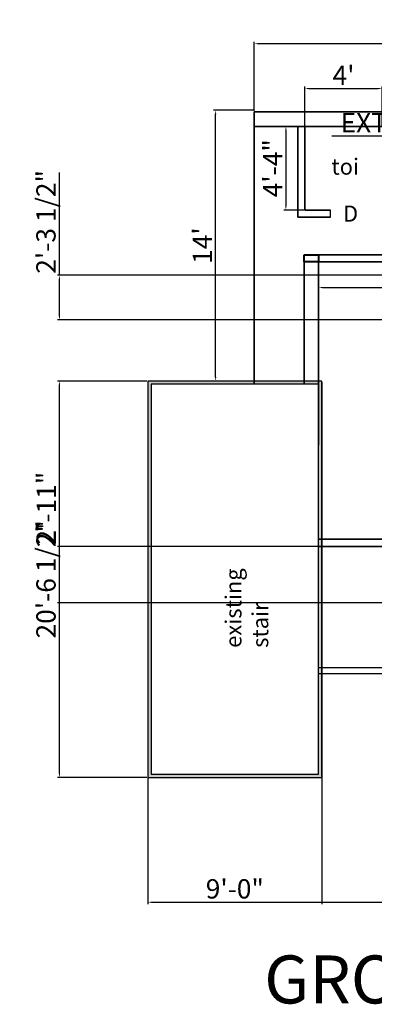
# Model space of a CAD drawing. Units: inches. Extents: x 1989 to 3287, y 1752 to 2384.
# Tile 1 of 5: x 1989 to 2209, y 1752 to 2364. Entities that reach past the tile are written whole.
import ezdxf

# ---------------------------------------------------------------- set-up
doc = ezdxf.new("R2010")
doc.units = ezdxf.units.IN
for name, color, linetype, lineweight in [('A-ANNO-DIMS', 2, 'Continuous', 18), ('A-ANNO-TEXT', 7, 'Continuous', 18), ('A-AREA-IDEN', 7, 'Continuous', 18), ('A-COLS', 1, 'Continuous', 40), ('A-COLS-PATT', 8, 'Continuous', 13), ('A-DOOR', 3, 'Continuous', 25), ('A-FLOR-EDGE', 7, 'Continuous', 25), ('A-FLOR-PATT', 252, 'Continuous', 13), ('A-FLOR-STRS', 7, 'Continuous', 25), ('A-WALL', 7, 'Continuous', 35)]:
    doc.layers.add(name, color=color, linetype=linetype, lineweight=lineweight)
doc.styles.get("Standard").update_dxf_attribs({"font": 'arial.ttf'})
doc.dimstyles.new('ISO-25', dxfattribs={"dimtxt": 12, "dimasz": 2.5, "dimexe": 1.25, "dimexo": 0.625, "dimtad": 1, "dimdec": 0, "dimlunit": 4, "dimtxsty": 'Standard', "dimcen": 2.5, "dimadec": 0, "dimazin": 0, "dimtfac": 1, "dimtdec": 0, "dimtmove": 0, "dimatfit": 3, "dimfxl": 1, "dimarcsym": 0})

# ---------------------------------------------------------------- blocks, each defined once
blk = doc.blocks.new('*D10')
at = {"layer": 'A-ANNO-DIMS', "color": 0, "lineweight": -2, "transparency": 16777216}
for p, q in [((2174.64, 2212.82), (2174.64, 2196.3)), ((2308.64, 2212.82), (2308.64, 2196.3)), ((2177.14, 2197.55), (2306.14, 2197.55))]:
    blk.add_line(p, q, dxfattribs=at)
at = {"layer": 'A-ANNO-DIMS', "color": 0, "transparency": 16777216}
for points in [[(2177.14, 2197.97), (2177.14, 2197.13), (2174.64, 2197.55)], [(2306.14, 2197.97), (2306.14, 2197.13), (2308.64, 2197.55)]]:
    blk.add_solid(points, dxfattribs=at)
at = {"layer": 'Defpoints', "color": 0, "transparency": 16777216}
for p in [(2174.64, 2213.45), (2308.64, 2213.45), (2308.64, 2197.55)]:
    blk.add_point(p, dxfattribs=at)
at = {"layer": 'A-ANNO-DIMS', "color": 0, "transparency": 16777216, "insert": (2241.64, 2204.2), "char_height": 12, "attachment_point": 5}
blk.add_mtext('11\'-2"', dxfattribs=at)
blk = doc.blocks.new('*D11')
at = {"layer": 'A-ANNO-DIMS', "color": 0, "lineweight": -2, "transparency": 16777216}
for p, q in [((2134.01, 2307.68), (2109.39, 2307.68)), ((2110.64, 2141.99), (2110.64, 2305.18)), ((2134.01, 2139.49), (2109.39, 2139.49))]:
    blk.add_line(p, q, dxfattribs=at)
at = {"layer": 'A-ANNO-DIMS', "color": 0, "transparency": 16777216}
for points in [[(2110.22, 2305.18), (2111.05, 2305.18), (2110.64, 2307.68)], [(2110.22, 2141.99), (2111.05, 2141.99), (2110.64, 2139.49)]]:
    blk.add_solid(points, dxfattribs=at)
at = {"layer": 'Defpoints', "color": 0, "transparency": 16777216}
for p in [(2110.64, 2307.68), (2134.64, 2307.68), (2134.64, 2139.49)]:
    blk.add_point(p, dxfattribs=at)
at = {"layer": 'A-ANNO-DIMS', "color": 0, "transparency": 16777216, "insert": (2103.99, 2223.59), "char_height": 12, "attachment_point": 5, "rotation": 90}
blk.add_mtext("14'", dxfattribs=at)
blk = doc.blocks.new('*D12')
at = {"layer": 'A-ANNO-DIMS', "color": 0, "lineweight": -2, "transparency": 16777216}
for p, q in [((2134.64, 2307.3), (2134.64, 2350.26)), ((2518.14, 2349.01), (2137.14, 2349.01)), ((2520.64, 2307.3), (2520.64, 2350.26))]:
    blk.add_line(p, q, dxfattribs=at)
at = {"layer": 'A-ANNO-DIMS', "color": 0, "transparency": 16777216}
for points in [[(2137.14, 2349.43), (2137.14, 2348.6), (2134.64, 2349.01)], [(2518.14, 2349.43), (2518.14, 2348.6), (2520.64, 2349.01)]]:
    blk.add_solid(points, dxfattribs=at)
at = {"layer": 'Defpoints', "color": 0, "transparency": 16777216}
for p in [(2134.64, 2349.01), (2134.64, 2306.68), (2520.64, 2306.68)]:
    blk.add_point(p, dxfattribs=at)
at = {"layer": 'A-ANNO-DIMS', "color": 0, "transparency": 16777216, "insert": (2327.64, 2355.77), "char_height": 12, "attachment_point": 5}
blk.add_mtext('32\'-2"', dxfattribs=at)
blk = doc.blocks.new('*D31')
at = {"layer": 'A-ANNO-DIMS', "color": 0, "lineweight": -2, "transparency": 16777216}
for p, q in [((2166.14, 2298.3), (2166.14, 2322.43)), ((2168.64, 2321.18), (2211.64, 2321.18)), ((2214.14, 2298.3), (2214.14, 2322.43))]:
    blk.add_line(p, q, dxfattribs=at)
at = {"layer": 'A-ANNO-DIMS', "color": 0, "transparency": 16777216}
for points in [[(2168.64, 2321.6), (2168.64, 2320.76), (2166.14, 2321.18)], [(2211.64, 2321.6), (2211.64, 2320.76), (2214.14, 2321.18)]]:
    blk.add_solid(points, dxfattribs=at)
at = {"layer": 'Defpoints', "color": 0, "transparency": 16777216}
for p in [(2214.14, 2321.18), (2166.14, 2297.68), (2214.14, 2297.68)]:
    blk.add_point(p, dxfattribs=at)
at = {"layer": 'A-ANNO-DIMS', "color": 0, "transparency": 16777216, "insert": (2190.14, 2327.8), "char_height": 12, "attachment_point": 5}
blk.add_mtext("4'", dxfattribs=at)
blk = doc.blocks.new('*D32')
at = {"layer": 'A-ANNO-DIMS', "color": 0, "lineweight": -2, "transparency": 16777216}
for p, q in [((2165.51, 2297.68), (2153.06, 2297.68)), ((2154.31, 2295.18), (2154.31, 2248.18)), ((2165.51, 2245.68), (2153.06, 2245.68))]:
    blk.add_line(p, q, dxfattribs=at)
at = {"layer": 'A-ANNO-DIMS', "color": 0, "transparency": 16777216}
for points in [[(2153.89, 2295.18), (2154.73, 2295.18), (2154.31, 2297.68)], [(2153.89, 2248.18), (2154.73, 2248.18), (2154.31, 2245.68)]]:
    blk.add_solid(points, dxfattribs=at)
at = {"layer": 'Defpoints', "color": 0, "transparency": 16777216}
for p in [(2166.14, 2297.68), (2154.31, 2245.68), (2166.14, 2245.68)]:
    blk.add_point(p, dxfattribs=at)
at = {"layer": 'A-ANNO-DIMS', "color": 0, "transparency": 16777216, "insert": (2147.68, 2271.68), "char_height": 12, "attachment_point": 5, "rotation": 90}
blk.add_mtext('4\'-4"', dxfattribs=at)
blk = doc.blocks.new('*D53')
at = {"layer": 'A-ANNO-DIMS', "color": 0, "lineweight": -2, "transparency": 16777216}
for p, q in [((2407.24, 2297.05), (2407.24, 2290.35)), ((2447.79, 2297.05), (2447.79, 2290.35)), ((2407.24, 2291.6), (2182.88, 2291.6)), ((2445.29, 2291.6), (2409.74, 2291.6))]:
    blk.add_line(p, q, dxfattribs=at)
at = {"layer": 'A-ANNO-DIMS', "color": 0, "transparency": 16777216}
for points in [[(2409.74, 2292.01), (2409.74, 2291.18), (2407.24, 2291.6)], [(2445.29, 2292.01), (2445.29, 2291.18), (2447.79, 2291.6)]]:
    blk.add_solid(points, dxfattribs=at)
at = {"layer": 'Defpoints', "color": 0, "transparency": 16777216}
for p in [(2407.24, 2297.68), (2447.79, 2297.68), (2407.24, 2291.6)]:
    blk.add_point(p, dxfattribs=at)
at = {"layer": 'A-ANNO-DIMS', "color": 0, "transparency": 16777216, "insert": (2293.81, 2298.44), "char_height": 12, "attachment_point": 5}
blk.add_mtext('EXT. WINDOW 3\'-4 1/2" TYP.', dxfattribs=at)
blk = doc.blocks.new('*D63')
at = {"layer": 'A-ANNO-DIMS', "color": 0, "lineweight": -2, "transparency": 16777216}
for p, q in [((2521.64, 2069.99), (2521.64, 1814.48)), ((2068.49, 1892.56), (2068.49, 1814.48)), ((2070.99, 1815.73), (2519.14, 1815.73))]:
    blk.add_line(p, q, dxfattribs=at)
at = {"layer": 'A-ANNO-DIMS', "color": 0, "transparency": 16777216}
for points in [[(2070.99, 1816.15), (2070.99, 1815.31), (2068.49, 1815.73)], [(2519.14, 1816.15), (2519.14, 1815.31), (2521.64, 1815.73)]]:
    blk.add_solid(points, dxfattribs=at)
at = {"layer": 'Defpoints', "color": 0, "transparency": 16777216}
for p in [(2521.64, 2070.62), (2068.49, 1893.19), (2521.64, 1815.73)]:
    blk.add_point(p, dxfattribs=at)
at = {"layer": 'A-ANNO-DIMS', "color": 0, "transparency": 16777216, "insert": (2295.06, 1822.49), "char_height": 12, "attachment_point": 5}
blk.add_mtext('37\'-9"', dxfattribs=at)
blk = doc.blocks.new('*D67')
at = {"layer": 'A-ANNO-DIMS', "color": 0, "lineweight": -2, "transparency": 16777216}
for p, q in [((2067.86, 2139.49), (2012.29, 2139.49)), ((2013.54, 1895.69), (2013.54, 2136.99)), ((2067.86, 1893.19), (2012.29, 1893.19))]:
    blk.add_line(p, q, dxfattribs=at)
at = {"layer": 'A-ANNO-DIMS', "color": 0, "transparency": 16777216}
for points in [[(2013.12, 2136.99), (2013.95, 2136.99), (2013.54, 2139.49)], [(2013.12, 1895.69), (2013.95, 1895.69), (2013.54, 1893.19)]]:
    blk.add_solid(points, dxfattribs=at)
at = {"layer": 'Defpoints', "color": 0, "transparency": 16777216}
for p in [(2013.54, 2139.49), (2068.49, 2139.49), (2068.49, 1893.19)]:
    blk.add_point(p, dxfattribs=at)
at = {"layer": 'A-ANNO-DIMS', "color": 0, "transparency": 16777216, "insert": (2006.71, 2016.34), "char_height": 12, "attachment_point": 5, "rotation": 90}
blk.add_mtext('20\'-6 1/2"', dxfattribs=at)
blk = doc.blocks.new('*D68')
at = {"layer": 'A-ANNO-DIMS', "color": 0, "lineweight": -2, "transparency": 16777216}
for p, q in [((2068.49, 2138.87), (2068.49, 1814.48)), ((2176.64, 2138.87), (2176.64, 1814.48)), ((2070.99, 1815.73), (2174.14, 1815.73))]:
    blk.add_line(p, q, dxfattribs=at)
at = {"layer": 'A-ANNO-DIMS', "color": 0, "transparency": 16777216}
for points in [[(2070.99, 1816.15), (2070.99, 1815.31), (2068.49, 1815.73)], [(2174.14, 1816.15), (2174.14, 1815.31), (2176.64, 1815.73)]]:
    blk.add_solid(points, dxfattribs=at)
at = {"layer": 'Defpoints', "color": 0, "transparency": 16777216}
for p in [(2068.49, 2139.49), (2176.64, 2139.49), (2176.64, 1815.73)]:
    blk.add_point(p, dxfattribs=at)
at = {"layer": 'A-ANNO-DIMS', "color": 0, "transparency": 16777216, "insert": (2122.56, 1822.48), "char_height": 12, "attachment_point": 5}
blk.add_mtext('9\'-0"', dxfattribs=at)
blk = doc.blocks.new('*D75')
at = {"layer": 'A-ANNO-DIMS', "color": 0, "lineweight": -2, "transparency": 16777216}
for p, q in [((2013.54, 2205.2), (2013.54, 2269.02)), ((2308.01, 2205.2), (2012.29, 2205.2)), ((2013.54, 2179.95), (2013.54, 2202.7)), ((2308.01, 2177.45), (2012.29, 2177.45))]:
    blk.add_line(p, q, dxfattribs=at)
at = {"layer": 'A-ANNO-DIMS', "color": 0, "transparency": 16777216}
for points in [[(2013.12, 2202.7), (2013.95, 2202.7), (2013.54, 2205.2)], [(2013.12, 2179.95), (2013.95, 2179.95), (2013.54, 2177.45)]]:
    blk.add_solid(points, dxfattribs=at)
at = {"layer": 'Defpoints', "color": 0, "transparency": 16777216}
for p in [(2013.54, 2205.2), (2308.64, 2205.2), (2308.64, 2177.45)]:
    blk.add_point(p, dxfattribs=at)
at = {"layer": 'A-ANNO-DIMS', "color": 0, "transparency": 16777216, "insert": (2006.7, 2238.36), "char_height": 12, "attachment_point": 5, "rotation": 90}
blk.add_mtext('2\'-3 1/2"', dxfattribs=at)
blk = doc.blocks.new('*D77')
at = {"layer": 'A-ANNO-DIMS', "color": 0, "lineweight": -2, "transparency": 16777216}
for p, q in [((2013.54, 2036.68), (2013.54, 2081.86)), ((2405.51, 2036.68), (2012.29, 2036.68)), ((2013.54, 2004.18), (2013.54, 2034.18)), ((2395.51, 2001.68), (2012.29, 2001.68))]:
    blk.add_line(p, q, dxfattribs=at)
at = {"layer": 'A-ANNO-DIMS', "color": 0, "transparency": 16777216}
for points in [[(2013.12, 2034.18), (2013.95, 2034.18), (2013.54, 2036.68)], [(2013.12, 2004.18), (2013.95, 2004.18), (2013.54, 2001.68)]]:
    blk.add_solid(points, dxfattribs=at)
at = {"layer": 'Defpoints', "color": 0, "transparency": 16777216}
for p in [(2013.54, 2036.68), (2406.14, 2036.68), (2396.14, 2001.68)]:
    blk.add_point(p, dxfattribs=at)
at = {"layer": 'A-ANNO-DIMS', "color": 0, "transparency": 16777216, "insert": (2006.89, 2060.52), "char_height": 12, "attachment_point": 5, "rotation": 90}
blk.add_mtext('2\'-11"', dxfattribs=at)

msp = doc.modelspace()

# ---------------------------------------------------------------- hatches: boundary and pattern name
at = {"layer": 'A-COLS-PATT'}
h = msp.add_hatch(dxfattribs=at)
h.set_pattern_fill('GRAVEL', color=256, scale=0.2)
h.paths.add_polyline_path([(2520.64, 2045.68), (2511.64, 2045.68), (2511.64, 2041.18), (2510.64, 2041.18), (2510.64, 2036.68), (2520.64, 2036.68)])
h.paths.add_polyline_path([(2520.63, 1966.68), (2510.63, 1966.68), (2510.63, 1957.68), (2520.63, 1957.68)])
h.paths.add_polyline_path([(2323.14, 1882.68), (2313.14, 1882.68), (2313.14, 1873.68), (2323.14, 1873.68)])
h.paths.add_polyline_path([(2378.64, 1882.68), (2368.64, 1882.68), (2368.64, 1873.68), (2378.64, 1873.68)])
h.paths.add_polyline_path([(2378.64, 1966.68), (2368.64, 1966.68), (2368.64, 1957.68), (2378.64, 1957.68)])
h.paths.add_polyline_path([(2323.14, 1966.68), (2313.14, 1966.68), (2313.14, 1957.68), (2323.14, 1957.68)])
h.paths.add_polyline_path([(2313.14, 2041.18), (2308.64, 2041.18), (2308.64, 2036.68), (2313.14, 2036.68)])
h.paths.add_polyline_path([(2304.29, 2102.44), (2304.29, 2151.15), (2279.56, 2151.15), (2279.56, 2102.44)], flags=9)
h.paths.add_polyline_path([(2216.76, 2191.62), (2265.47, 2191.62), (2265.47, 2216.35), (2216.76, 2216.35)], flags=9)
h.paths.add_polyline_path([(2507.53, 2217.24), (2507.53, 2245.08), (2482.8, 2245.08), (2482.8, 2217.24)], flags=9)
h.paths.add_polyline_path([(2466.45, 2144.02), (2484.98, 2144.02), (2484.98, 2168.75), (2466.45, 2168.75)], flags=9)
h.paths.add_polyline_path([(2462.3, 2086.74), (2462.3, 2114.58), (2437.57, 2114.58), (2437.57, 2086.74)], flags=9)
h.paths.add_polyline_path([(2349.26, 2050.52), (2397.97, 2050.52), (2397.97, 2075.25), (2349.26, 2075.25)], flags=9)
h.paths.add_polyline_path([(2432.27, 2086.74), (2432.27, 2114.58), (2407.54, 2114.58), (2407.54, 2086.74)], flags=9)
h.paths.add_polyline_path([(2304.67, 2184.6), (2319.75, 2184.6), (2319.75, 2205.2), (2304.67, 2205.2)], flags=9)
h.paths.add_polyline_path([(2345.88, 2187.62), (2360.97, 2187.62), (2360.97, 2208.22), (2345.88, 2208.22)], flags=9)
h.paths.add_polyline_path([(2429.95, 2091.23), (2445.03, 2091.23), (2445.03, 2111.84), (2429.95, 2111.84)], flags=9)
h.paths.add_polyline_path([(2346.78, 2233.62), (2361.86, 2233.62), (2361.86, 2254.22), (2346.78, 2254.22)], flags=9)
h.paths.add_polyline_path([(2222.31, 2236.18), (2237.39, 2236.18), (2237.39, 2256.78), (2222.31, 2256.78)], flags=9)
h.paths.add_polyline_path([(2186.25, 2233.03), (2201.34, 2233.03), (2201.34, 2253.64), (2186.25, 2253.64)], flags=9)
h.paths.add_polyline_path([(2356.5, 2089.75), (2417.39, 2089.75), (2417.39, 2110.36), (2356.5, 2110.36)], flags=9)
h.paths.add_polyline_path([(2450.78, 2087.89), (2500.04, 2087.89), (2500.04, 2108.49), (2450.78, 2108.49)], flags=9)
h.paths.add_polyline_path([(2226.77, 2120.65), (2286.89, 2120.65), (2286.89, 2141.25), (2226.77, 2141.25)], flags=9)
h.paths.add_polyline_path([(2422.03, 2219.06), (2486.03, 2219.06), (2486.03, 2239.67), (2422.03, 2239.67)], flags=9)
h.paths.add_polyline_path([(2321.5, 2262.24), (2341.25, 2262.24), (2341.25, 2282.84), (2321.5, 2282.84)], flags=9)
h.paths.add_polyline_path([(2234.58, 2262.24), (2266.77, 2262.24), (2266.77, 2282.84), (2234.58, 2282.84)], flags=9)
h.paths.add_polyline_path([(2179.85, 2262.24), (2199.6, 2262.24), (2199.6, 2282.84), (2179.85, 2282.84)], flags=9)
at = {"layer": 'A-FLOR-PATT'}
h = msp.add_hatch(color=256, dxfattribs=at)
h.dxf.hatch_style = 1
h.paths.add_polyline_path([(2134.64, 2139.49), (2068.49, 2139.49), (2068.49, 1893.19), (2176.64, 1893.19), (2176.64, 2139.49), (2174.64, 2139.49), (2174.64, 2099.68), (2174.64, 1895.19), (2070.49, 1895.19), (2070.49, 2137.49), (2134.64, 2137.49)])
h.paths.add_polyline_path([(2165.64, 2139.49), (2134.64, 2139.49), (2134.64, 2137.49), (2165.64, 2137.49)], flags=17)
h.paths.add_polyline_path([(2174.64, 2139.49), (2165.64, 2139.49), (2165.64, 2137.49), (2174.64, 2137.49)], flags=17)

# ---------------------------------------------------------------- linework, layer by layer
at = {"layer": 'A-COLS'}
msp.add_lwpolyline([(2165.64, 2217.95), (2174.64, 2217.95), (2174.64, 2213.45), (2165.64, 2213.45)], close=True, dxfattribs=at)
at = {"layer": 'A-DOOR'}
msp.add_line((2182.14, 2241.18), (2182.14, 2245.68), dxfattribs=at)
at = {"layer": 'A-FLOR-EDGE'}
for p, q in [((2174.64, 1961.55), (2313.14, 1961.55)), ((2312.64, 1957.68), (2174.64, 1957.68))]:
    msp.add_line(p, q, dxfattribs=at)
at = {"layer": 'A-FLOR-STRS'}
for points in [[(2176.64, 2139.49), (2068.49, 2139.49), (2068.49, 1893.19), (2176.64, 1893.19)], [(2174.64, 2137.49), (2070.49, 2137.49), (2070.49, 1895.19), (2174.64, 1895.19)]]:
    msp.add_lwpolyline(points, close=True, dxfattribs=at)
at = {"layer": 'A-WALL'}
for p, q in [((2143.64, 2297.68), (2134.64, 2297.68)), ((2161.64, 2297.68), (2161.64, 2241.18)), ((2214.14, 2297.68), (2166.14, 2297.68)), ((2166.14, 2297.68), (2166.14, 2245.68)), ((2166.14, 2245.68), (2182.14, 2245.68)), ((2161.64, 2241.18), (2182.14, 2241.18)), ((2165.64, 2137.49), (2165.64, 2217.95)), ((2313.14, 2217.95), (2165.64, 2217.95)), ((2174.64, 2099.68), (2174.64, 2213.45)), ((2308.64, 2213.45), (2174.64, 2213.45)), ((2299.29, 2041.18), (2174.64, 2041.18)), ((2302.64, 2036.68), (2174.64, 2036.68))]:
    msp.add_line(p, q, dxfattribs=at)
for points in [[(2520.64, 2090.68), (2520.64, 2306.68), (2134.64, 2306.68), (2134.64, 2137.49)], [(2511.64, 2099.68), (2511.64, 2297.68), (2143.64, 2297.68)]]:
    msp.add_lwpolyline(points, dxfattribs=at)

# ---------------------------------------------------------------- texts
at = {"layer": 'A-ANNO-TEXT', "attachment_point": 1}
for s, width, gutter_width, insert, char_height in [('D', 78.3523, 49.99, (2189.83, 2248.49), 10), ('GROUND FLOOR', 4273.6475, 149.09, (2140.81, 1782.67), 29.8187)]:
    msp.add_mtext_dynamic_manual_height_columns(s, width=width, gutter_width=gutter_width, heights=[0], dxfattribs=dict(at, insert=insert, char_height=char_height))
at = {"layer": 'A-ANNO-TEXT', "insert": (2116.68, 1973.76), "char_height": 9.9978, "attachment_point": 1, "rotation": 90}
msp.add_mtext_dynamic_manual_height_columns('existing stair', width=78.3523, gutter_width=49.99, heights=[0], dxfattribs=at)
at = {"layer": 'A-AREA-IDEN', "insert": (2182.6, 2277.69), "char_height": 9.998, "attachment_point": 1}
msp.add_mtext_dynamic_manual_height_columns('toi', width=78.3523, gutter_width=49.99, heights=[0], dxfattribs=at)

# ---------------------------------------------------------------- dimensions: what is measured, and where the dimension line sits
at = {"layer": 'A-ANNO-DIMS'}
for base, p1, p2, override, picture, middle in [((2134.64, 2349.01), (2520.64, 2306.68), (2134.64, 2306.68), {"dimclrd": 0, "dimclre": 0, "dimclrt": 0}, '*D12', (2327.64, 2355.77)), ((2214.14, 2321.18), (2166.14, 2297.68), (2214.14, 2297.68), {"dimclrd": 0, "dimclre": 0, "dimclrt": 0}, '*D31', (2190.14, 2327.8)), ((2308.64, 2197.55), (2174.64, 2213.45), (2308.64, 2213.45), {"dimclrd": 0, "dimclre": 0, "dimclrt": 0}, '*D10', (2241.64, 2204.2)), ((2176.6365, 1815.73), (2068.4852, 2139.4944), (2176.6365, 2139.4944), {"dimdec": 1, "dimlfac": 1, "dimrnd": 0, "dimzin": 1, "dimdsep": 46, "dimlunit": 4, "dimfrac": 2}, '*D68', (2122.5609, 1822.4819)), ((2521.6365, 1815.73), (2068.4852, 1893.1857), (2521.6365, 2070.6179), {"dimdec": 1, "dimlfac": 1, "dimrnd": 0, "dimzin": 1, "dimdsep": 46, "dimlunit": 4, "dimfrac": 2}, '*D63', (2295.0609, 1822.486))]:
    dim = msp.add_linear_dim(base=base, p1=p1, p2=p2, dimstyle='ISO-25', override=override, dxfattribs=at)
    dim.commit()
    dim.dimension.update_dxf_attribs({"geometry": picture, "text_midpoint": middle})
dim = msp.add_linear_dim(base=(2407.2411, 2291.5978), p1=(2447.789, 2297.68), p2=(2407.2411, 2297.68), angle=180, text='EXT. WINDOW <> TYP.', dimstyle='ISO-25', override={"dimdec": 1, "dimlfac": 1, "dimrnd": 0, "dimzin": 1, "dimdsep": 46, "dimlunit": 4, "dimfrac": 2}, dxfattribs=at)
dim.commit()
dim.dimension.update_dxf_attribs({"geometry": '*D53', "text_midpoint": (2293.8119, 2298.4356)})
for base, p1, p2, override, picture, middle in [((2110.64, 2307.68), (2134.64, 2139.49), (2134.64, 2307.68), {"dimclrd": 0, "dimclre": 0, "dimclrt": 0}, '*D11', (2103.99, 2223.59)), ((2154.31, 2245.68), (2166.14, 2297.68), (2166.14, 2245.68), {"dimclrd": 0, "dimclre": 0, "dimclrt": 0}, '*D32', (2147.68, 2271.68)), ((2013.5352, 2205.2028), (2308.6365, 2177.4539), (2308.6365, 2205.2028), {"dimdec": 1, "dimlfac": 1, "dimrnd": 0, "dimzin": 1, "dimdsep": 46, "dimlunit": 4, "dimfrac": 2}, '*D75', (2006.7015, 2238.3605)), ((2013.54, 2139.49), (2068.49, 1893.19), (2068.49, 2139.49), {"dimdec": 1, "dimlfac": 1, "dimrnd": 0, "dimzin": 1, "dimdsep": 46, "dimlunit": 4, "dimfrac": 2}, '*D67', (2006.71, 2016.34)), ((2013.54, 2036.68), (2396.14, 2001.68), (2406.14, 2036.68), {"dimdec": 1, "dimlfac": 1, "dimrnd": 0, "dimzin": 1, "dimdsep": 46, "dimlunit": 4, "dimfrac": 2}, '*D77', (2006.89, 2060.52))]:
    dim = msp.add_linear_dim(base=base, p1=p1, p2=p2, angle=90, dimstyle='ISO-25', override=override, dxfattribs=at)
    dim.commit()
    dim.dimension.update_dxf_attribs({"geometry": picture, "text_midpoint": middle})

doc.saveas('drawing.dxf')
